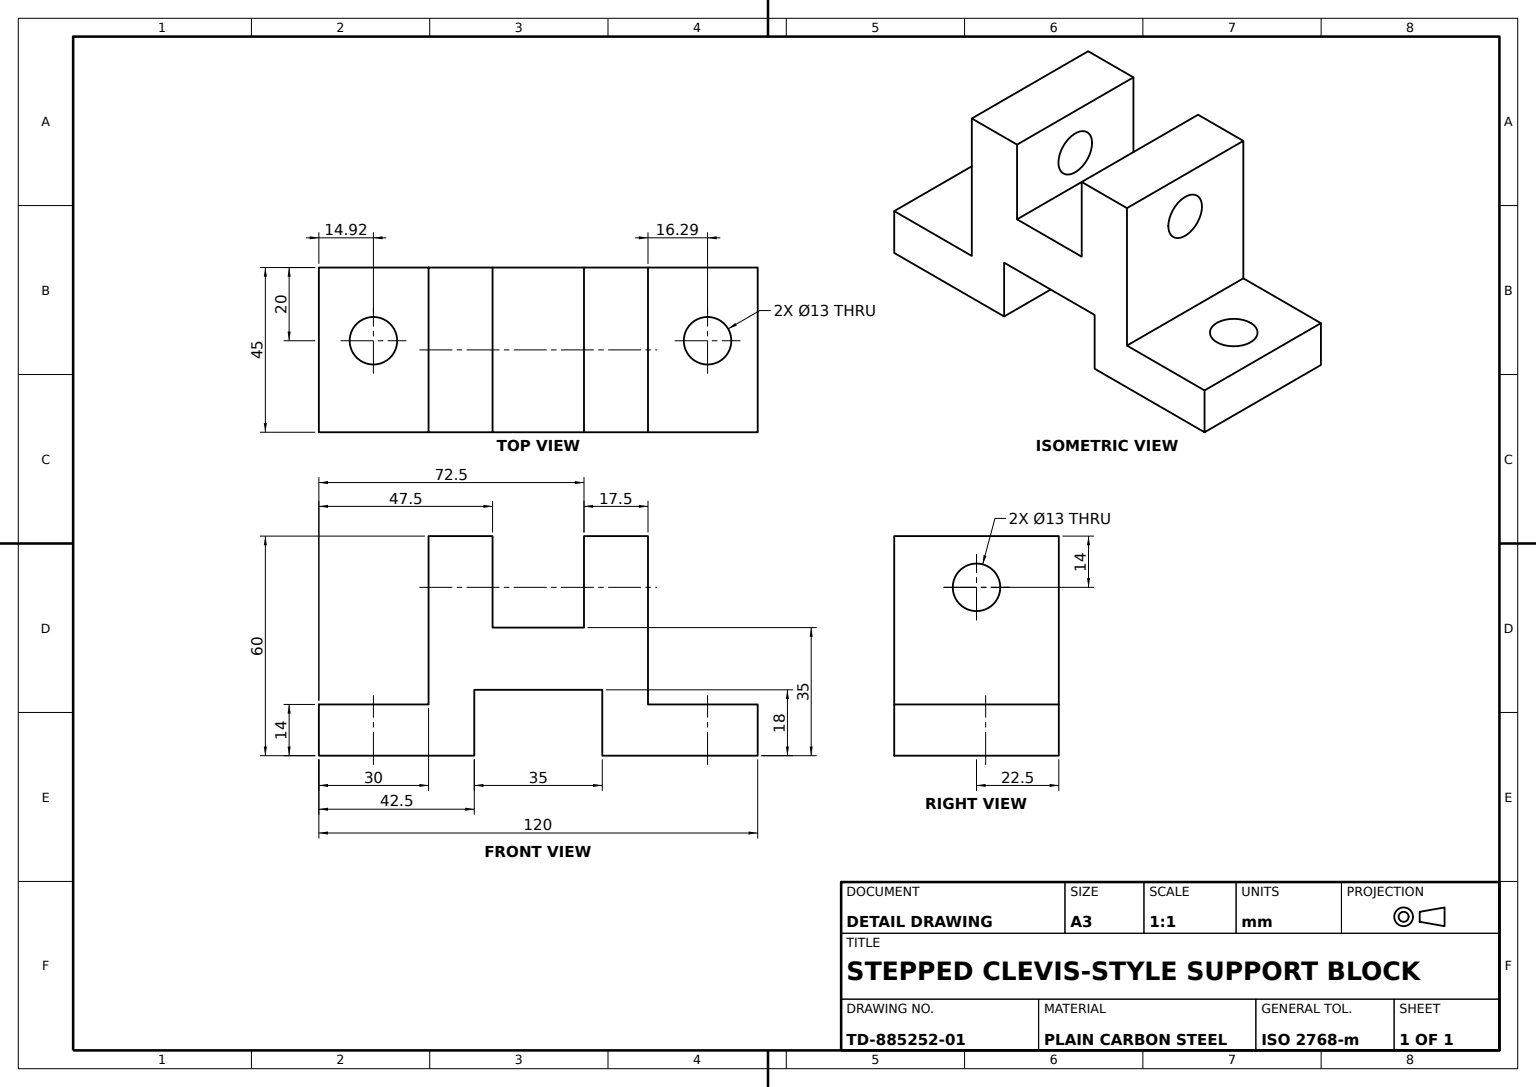
SolidWorks part; units mm, degrees
material "Plain Carbon Steel"
ref_plane "Front Plane" through (0, 0, 0) normal (0, 0, 1) x (1, 0, 0)
ref_plane "Top Plane" through (0, 0, 0) normal (0, 1, 0) x (1, 0, 0)
ref_plane "Right Plane" through (0, 0, 0) normal (1, 0, 0) x (0, 0, -1)
sketch "Bracket Profile Sketch" plane through (0, 0, 0) normal (0, 0, 1) x (1, 0, 0)
  line L0 (0, 0) -> (42.5, 0)
  line L1 (42.5, 0) -> (42.5, 18)
  line L2 (42.5, 18) -> (77.5, 18)
  line L3 (77.5, 18) -> (77.5, 0)
  line L4 (77.5, 0) -> (120, 0)
  line L5 (120, 0) -> (120, 14)
  line L6 (120, 14) -> (90, 14)
  line L7 (90, 14) -> (90, 60)
  line L8 (90, 60) -> (72.5, 60)
  line L9 (72.5, 60) -> (72.5, 35)
  line L10 (72.5, 35) -> (47.5, 35)
  line L11 (47.5, 35) -> (47.5, 60)
  line L12 (47.5, 60) -> (30, 60)
  line L13 (30, 60) -> (30, 14)
  line L14 (30, 14) -> (0, 14)
  line L15 (0, 14) -> (0, 0)
  dimension "D1" = 30
  dimension "D2" = 42.5
  dimension "D3" = 47.5
  dimension "D4" = 72.5
  dimension "D5" = 14
  dimension "D6" = 18
  dimension "D7" = 35
extrude "Bracket Body" add sketch "Bracket Profile Sketch" along normal blind 45
sketch "Upright Hole A Sketch" plane through (30, 0, 0) normal (-1, 0, 0) x (0, 0, 1)
  line L0 (45, 60) -> (0, 60) construction
  line L1 (45, 60) -> (45, 14) construction
  circle A0 centre (22.5, 46) radius 6.5
  dimension "D1" = 13
  dimension "D4" = 13
  dimension "D2" = 14
  dimension "D3" = 22.5
extrude "Upright Hole A Ø13" cut sketch "Upright Hole A Sketch" against normal blind 17.5
sketch "Upright Hole B Sketch" plane through (90, 0, 0) normal (1, 0, 0) x (0, 0, -1)
  line L0 (-45, 60) -> (0, 60) construction
  line L1 (0, 14) -> (0, 60) construction
  circle A0 centre (-22.5, 46) radius 6.5
  dimension "D1" = 13
  dimension "D4" = 13
  dimension "D2" = 14
  dimension "D3" = 22.5
extrude "Upright Hole B Ø13" cut sketch "Upright Hole B Sketch" against normal blind 17.5
sketch "Flange Hole A Sketch" plane through (0, 14, 0) normal (0, 1, 0) x (1, 0, 0)
  line L0 (30, 0) -> (0, 0) construction
  line L1 (0, -45) -> (0, 0) construction
  circle A0 centre (14.9197, -20) radius 6.5
  dimension "D1" = 13
  dimension "D3" = 13
  dimension "D2" = 20
  dimension "D4" = 14.9197
extrude "Flange Hole A Ø13" cut sketch "Flange Hole A Sketch" against normal blind 14
sketch "Flange Hole B Sketch" plane through (0, 14, 0) normal (0, 1, 0) x (1, 0, 0)
  line L0 (120, 0) -> (90, 0) construction
  line L1 (90, -45) -> (90, 0) construction
  circle A0 centre (106.2879, -20) radius 6.5
  dimension "D1" = 13
  dimension "D3" = 13
  dimension "D2" = 20
  dimension "D4" = 16.2879
extrude "Flange Hole B Ø13" cut sketch "Flange Hole B Sketch" against normal blind 14
